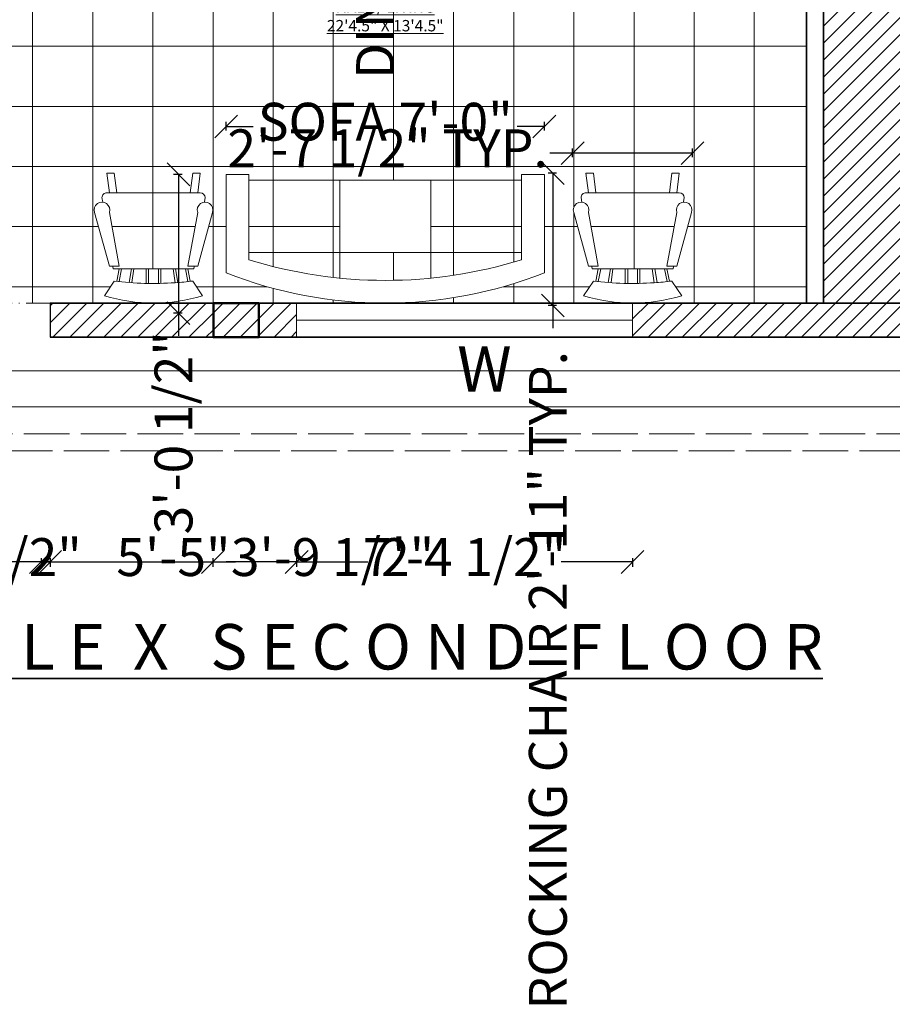
# Model space of a CAD drawing. Units: inches. Extents: x 2036 to 2670, y 319 to 920.
# Tile 2 of 15: x 2219 to 2449, y 319 to 579. Entities that reach past the tile are written whole.
import ezdxf

# ---------------------------------------------------------------- set-up
doc = ezdxf.new("R2010")
doc.units = ezdxf.units.IN
doc.linetypes.add('ACAD_ISO02W100', pattern=[15, 12, -3])
doc.linetypes.add('ACAD_ISO06W100', pattern=[36, 24, -3, 0, -3, 0, -3, 0, -3])
for name, color, linetype, lineweight in [('A-ANNO-DIMS', 2, 'Continuous', 18), ('A-ANNO-TEXT', 7, 'Continuous', 18), ('A-ANNO-TITL', 7, 'Continuous', 35), ('A-AREA-IDEN', 7, 'Continuous', 18), ('A-CASE-PATT', 9, 'Continuous', 13), ('A-COLS', 7, 'Continuous', 50), ('A-DOOR', 3, 'Continuous', 25), ('A-DOOR-OVHD', 3, 'ACAD_ISO06W100', 18), ('A-FLOR-OVHD', 1, 'ACAD_ISO02W100', 13), ('A-FLOR-PATT', 8, 'Continuous', 9), ('A-FURN', 8, 'Continuous', 18), ('A-GLAZ', 4, 'Continuous', 18), ('A-WALL', 7, 'Continuous', 35)]:
    doc.layers.add(name, color=color, linetype=linetype, lineweight=lineweight)
doc.layers.add('A-COLS-PATT', color=240, linetype='Continuous', lineweight=13, true_color=0xed1f24)
doc.layers.add('A-WALL-PATT', color=52, linetype='Continuous', lineweight=13, true_color=0xc8c92d)
doc.styles.get("Standard").update_dxf_attribs({"font": 'arial.ttf'})
doc.dimstyles.new('ISO-25', dxfattribs={"dimtxt": 10, "dimasz": 6, "dimexe": 1.25, "dimexo": 0.625, "dimtad": 0, "dimdec": 1, "dimlunit": 3, "dimtxsty": 'Standard', "dimblk": 'OBLIQUE', "dimcen": 2.5, "dimclrd": 94, "dimclre": 94, "dimclrt": 1, "dimadec": 0, "dimazin": 0, "dimtfac": 1, "dimtdec": 1, "dimtmove": 0, "dimatfit": 3, "dimfxl": 1, "dimfxlon": 1, "dimarcsym": 0})

# ---------------------------------------------------------------- blocks, each defined once
blk = doc.blocks.new('Chair - Rocking')
for p, q in [((-8, -4.5), (-10, -1.5)), ((8, -4.5), (10, -1.5)), ((-7.5, -4.5), (-7, -7)), ((-6.5, -7), (-7.02225, -4.43)), ((-4.5, -7), (-4.96674, -4.19951)), ((-4, -7), (-4.40532, -4.16272)), ((-1.5, -4.05012), (-1.5, -7)), ((-1, -7), (-1, -4.05012)), ((1, -7), (1, -4.04655)), ((1.5, -4.05012), (1.5, -7)), ((4, -7), (4.40187, -4.18694)), ((4.5, -7), (4.96761, -4.19437)), ((6.5, -7), (7, -4.4057)), ((7.5, -4.5), (7, -7)), ((-9, -7.5), (-12, -18.49999)), ((-7, -7.5), (-9, -7.5)), ((-9, -18.49999), (-7, -7.5)), ((-8.23428, -6.99939), (-8.3093, -7.47958)), ((-8.23041, -7), (8.23915, -7)), ((7, -7.5), (9, -7.5)), ((9, -18.49999), (7, -7.5)), ((8.31071, -7.48854), (8.23449, -7.00073)), ((9, -7.5), (12, -18.49999)), ((-10.36644, -20.64523), (-10.5, -21.49999)), ((10.5, -21.49999), (10.3575, -20.58798)), ((-9, -22.49999), (-9.5, -26.49999)), ((0, -22.49999), (-9.5, -22.49999)), ((-8, -26.49999), (-7.5, -22.49999)), ((0, -22.49999), (9.5, -22.49999)), ((8, -26.49999), (7.5, -22.49999)), ((9, -22.49999), (9.5, -26.49999)), ((-9.5, -26.49999), (-8, -26.49999)), ((9.5, -26.49999), (8, -26.49999))]:
    blk.add_line(p, q)
for centre, radius, start, end in [((0, -34.08333), 34.08333, 72.93847, 107.0615), ((0, -68.25004), 64.25, 82.84733, 93.92211), ((0, -68.25004), 64.25, 93.92211, 97.15267), ((-10.5, -18.99999), 1.58114, 161.5651, 18.43495), ((10.5, -18.99999), 1.58114, 161.5651, 18.43495), ((-9.5, -21.49999), 1, 180, 270), ((9.5, -21.49999), 1, 270, 0)]:
    blk.add_arc(centre, radius, start, end)
blk = doc.blocks.new('Sofa - Roundback 7 ft.')
for p, q in [((-12.00002, -32.4421), (-12.00003, -6.5971)), ((11.99997, -32.4421), (11.99998, -6.5971)), ((-36.000027, -34), (-36.000027, -11.4696)), ((35.99998, -34), (35.99998, -11.4696)), ((-35.999844, -13.3819), (35.9998, -13.3819)), ((-36.000027, -32.4421), (35.99998, -32.4421))]:
    blk.add_line(p, q)
for points in [[(-36.000027, -34), (-42.000027, -34), (-42.000027, -8)], [(41.99998, -8), (41.99998, -34), (35.99998, -34)]]:
    blk.add_lwpolyline(points)
for centre, radius, start, end in [((0, -114.25), 114.25, 68.43141, 111.5686), ((-0.00001, -127.1968), 121.1968, 72.72033, 107.2797)]:
    blk.add_arc(centre, radius, start, end)
blk = doc.blocks.new('COL-9x12')
blk.add_lwpolyline([(9, 0), (0, 0), (0, 12), (9, 12)], close=True)
blk = doc.blocks.new('_Oblique')
at = {"color": 0, "linetype": 'ByBlock', "lineweight": -2}
blk.add_line((-0.5, -0.5), (0.5, 0.5), dxfattribs=at)
blk = doc.blocks.new('*D25')
at = {"layer": 'A-ANNO-DIMS', "color": 94, "lineweight": -2, "transparency": 16777216}
for p, q in [((2360.81, 538.02), (2358.56, 538.02)), ((2359.81, 538.02), (2359.81, 503.04)), ((2360.81, 503.04), (2358.56, 503.04)), ((2359.81, 503.04), (2359.81, 497.04))]:
    blk.add_line(p, q, dxfattribs=at)
at = {"layer": 'Defpoints', "color": 0, "transparency": 16777216}
for p in [(2365.06, 538.02), (2359.81, 503.04), (2365.06, 503.04)]:
    blk.add_point(p, dxfattribs=at)
at = {"layer": 'A-ANNO-DIMS', "color": 94, "lineweight": -2, "transparency": 16777216, "xscale": 6, "yscale": 6, "zscale": 6}
for p, rotation in [((2359.81, 538.02), 90), ((2359.81, 503.04), 270)]:
    blk.add_blockref('_Oblique', p, dxfattribs=dict(at, rotation=rotation))
at = {"layer": 'A-ANNO-DIMS', "color": 1, "transparency": 16777216, "insert": (2359.81, 404.1), "char_height": 10, "attachment_point": 5, "rotation": 90}
blk.add_mtext('ROCKING CHAIR 2\'-11" TYP.', dxfattribs=at)
blk = doc.blocks.new('*D26')
at = {"layer": 'A-ANNO-DIMS', "color": 94, "lineweight": -2, "transparency": 16777216}
for p, q in [((2365.06, 542.26), (2365.06, 544.51)), ((2396.72, 542.26), (2396.72, 544.51)), ((2365.06, 543.26), (2359.06, 543.26)), ((2396.72, 543.26), (2365.06, 543.26))]:
    blk.add_line(p, q, dxfattribs=at)
at = {"layer": 'Defpoints', "color": 0, "transparency": 16777216}
for p in [(2365.06, 543.26), (2365.06, 538.02), (2396.72, 538.02)]:
    blk.add_point(p, dxfattribs=at)
at = {"layer": 'A-ANNO-DIMS', "color": 94, "lineweight": -2, "transparency": 16777216, "xscale": 6, "yscale": 6, "zscale": 6, "rotation": 180}
blk.add_blockref('_Oblique', (2365.06, 543.26), dxfattribs=at)
at = {"layer": 'A-ANNO-DIMS', "color": 94, "lineweight": -2, "transparency": 16777216, "xscale": 6, "yscale": 6, "zscale": 6}
blk.add_blockref('_Oblique', (2396.72, 543.26), dxfattribs=at)
at = {"layer": 'A-ANNO-DIMS', "color": 1, "transparency": 16777216, "insert": (2316.22, 543.26), "char_height": 10, "attachment_point": 5}
blk.add_mtext('2\'-7 1/2" TYP.', dxfattribs=at)
blk = doc.blocks.new('*D33')
at = {"layer": 'A-ANNO-DIMS', "color": 94, "lineweight": -2, "transparency": 16777216}
for p, q in [((2273.59, 549.28), (2273.59, 551.53)), ((2357.59, 549.28), (2357.59, 551.53)), ((2273.59, 550.28), (2280.74, 550.28)), ((2357.59, 550.28), (2350.44, 550.28))]:
    blk.add_line(p, q, dxfattribs=at)
at = {"layer": 'Defpoints', "color": 0, "transparency": 16777216}
for p in [(2273.59, 550.28), (2273.59, 537.68), (2357.59, 537.68)]:
    blk.add_point(p, dxfattribs=at)
at = {"layer": 'A-ANNO-DIMS', "color": 94, "lineweight": -2, "transparency": 16777216, "xscale": 6, "yscale": 6, "zscale": 6, "rotation": 180}
blk.add_blockref('_Oblique', (2273.59, 550.28), dxfattribs=at)
at = {"layer": 'A-ANNO-DIMS', "color": 94, "lineweight": -2, "transparency": 16777216, "xscale": 6, "yscale": 6, "zscale": 6}
blk.add_blockref('_Oblique', (2357.59, 550.28), dxfattribs=at)
at = {"layer": 'A-ANNO-DIMS', "color": 1, "transparency": 16777216, "insert": (2315.59, 550.28), "char_height": 10, "attachment_point": 5}
blk.add_mtext('SOFA 7\'-0"', dxfattribs=at)
blk = doc.blocks.new('*D34')
at = {"layer": 'A-ANNO-DIMS', "color": 94, "lineweight": -2, "transparency": 16777216}
for p, q in [((2261.99, 537.68), (2259.74, 537.68)), ((2260.99, 537.68), (2260.99, 501.02)), ((2261.99, 501.02), (2259.74, 501.02)), ((2260.99, 501.02), (2260.99, 495.02))]:
    blk.add_line(p, q, dxfattribs=at)
at = {"layer": 'Defpoints', "color": 0, "transparency": 16777216}
for p in [(2273.59, 537.68), (2260.99, 501.02), (2273.59, 501.02)]:
    blk.add_point(p, dxfattribs=at)
at = {"layer": 'A-ANNO-DIMS', "color": 94, "lineweight": -2, "transparency": 16777216, "xscale": 6, "yscale": 6, "zscale": 6}
for p, rotation in [((2260.99, 537.68), 90), ((2260.99, 501.02), 270)]:
    blk.add_blockref('_Oblique', p, dxfattribs=dict(at, rotation=rotation))
at = {"layer": 'A-ANNO-DIMS', "color": 1, "transparency": 16777216, "insert": (2260.99, 469.45), "char_height": 10, "attachment_point": 5, "rotation": 90}
blk.add_mtext('3\'-0 1/2"', dxfattribs=at)
blk = doc.blocks.new('*D39')
at = {"layer": 'A-ANNO-DIMS', "color": 94, "lineweight": -2, "transparency": 16777216}
for p, q in [((2315.21, 769.01), (2312.96, 769.01)), ((2314.21, 769.01), (2314.21, 678.01)), ((2315.21, 678.01), (2312.96, 678.01)), ((2314.21, 678.01), (2314.21, 672.01))]:
    blk.add_line(p, q, dxfattribs=at)
at = {"layer": 'Defpoints', "color": 0, "transparency": 16777216}
for p in [(2327.86, 769.01), (2314.21, 678.01), (2327.86, 678.01)]:
    blk.add_point(p, dxfattribs=at)
at = {"layer": 'A-ANNO-DIMS', "color": 94, "lineweight": -2, "transparency": 16777216, "xscale": 6, "yscale": 6, "zscale": 6}
for p, rotation in [((2314.21, 769.01), 90), ((2314.21, 678.01), 270)]:
    blk.add_blockref('_Oblique', p, dxfattribs=dict(at, rotation=rotation))
at = {"layer": 'A-ANNO-DIMS', "color": 1, "transparency": 16777216, "insert": (2314.21, 616.43), "char_height": 10, "attachment_point": 5, "rotation": 90}
blk.add_mtext('DINING SET 7\'-7"', dxfattribs=at)
blk = doc.blocks.new('*D41')
at = {"layer": 'A-ANNO-DIMS', "color": 94, "lineweight": -2, "transparency": 16777216}
for p, q in [((2149.74, 436.33), (2149.74, 434.08)), ((2149.74, 435.33), (2177.02, 435.33)), ((2177.02, 436.33), (2177.02, 434.08)), ((2177.02, 435.33), (2183.02, 435.33))]:
    blk.add_line(p, q, dxfattribs=at)
at = {"layer": 'Defpoints', "color": 0, "transparency": 16777216}
for p in [(2149.74, 494.68), (2177.02, 494.68), (2177.02, 435.33)]:
    blk.add_point(p, dxfattribs=at)
at = {"layer": 'A-ANNO-DIMS', "color": 94, "lineweight": -2, "transparency": 16777216, "xscale": 6, "yscale": 6, "zscale": 6, "rotation": 180}
blk.add_blockref('_Oblique', (2149.74, 435.33), dxfattribs=at)
at = {"layer": 'A-ANNO-DIMS', "color": 94, "lineweight": -2, "transparency": 16777216, "xscale": 6, "yscale": 6, "zscale": 6}
blk.add_blockref('_Oblique', (2177.02, 435.33), dxfattribs=at)
at = {"layer": 'A-ANNO-DIMS', "color": 1, "transparency": 16777216, "insert": (2208.67, 435.33), "char_height": 10, "attachment_point": 5}
blk.add_mtext('2\'-3 1/2"', dxfattribs=at)
blk = doc.blocks.new('*D42')
at = {"layer": 'A-ANNO-DIMS', "color": 94, "lineweight": -2, "transparency": 16777216}
for p, q in [((2177.02, 436.33), (2177.02, 434.08)), ((2177.02, 435.33), (2187.98, 435.33)), ((2227.17, 435.33), (2216.21, 435.33)), ((2227.17, 436.33), (2227.17, 434.08))]:
    blk.add_line(p, q, dxfattribs=at)
at = {"layer": 'Defpoints', "color": 0, "transparency": 16777216}
for p in [(2177.02, 494.68), (2227.17, 494.68), (2227.17, 435.33)]:
    blk.add_point(p, dxfattribs=at)
at = {"layer": 'A-ANNO-DIMS', "color": 94, "lineweight": -2, "transparency": 16777216, "xscale": 6, "yscale": 6, "zscale": 6, "rotation": 180}
blk.add_blockref('_Oblique', (2177.02, 435.33), dxfattribs=at)
at = {"layer": 'A-ANNO-DIMS', "color": 94, "lineweight": -2, "transparency": 16777216, "xscale": 6, "yscale": 6, "zscale": 6}
blk.add_blockref('_Oblique', (2227.17, 435.33), dxfattribs=at)
at = {"layer": 'A-ANNO-DIMS', "color": 1, "transparency": 16777216, "insert": (2202.09, 435.33), "char_height": 10, "attachment_point": 5}
blk.add_mtext('4\'-2"', dxfattribs=at)
blk = doc.blocks.new('*D43')
at = {"layer": 'A-ANNO-DIMS', "color": 94, "lineweight": -2, "transparency": 16777216}
for p, q in [((2227.17, 436.33), (2227.17, 434.08)), ((2227.17, 435.33), (2245.77, 435.33)), ((2292.21, 435.33), (2273.61, 435.33)), ((2292.21, 436.33), (2292.21, 434.08))]:
    blk.add_line(p, q, dxfattribs=at)
at = {"layer": 'Defpoints', "color": 0, "transparency": 16777216}
for p in [(2227.17, 494.68), (2292.21, 494.68), (2292.21, 435.33)]:
    blk.add_point(p, dxfattribs=at)
at = {"layer": 'A-ANNO-DIMS', "color": 94, "lineweight": -2, "transparency": 16777216, "xscale": 6, "yscale": 6, "zscale": 6, "rotation": 180}
blk.add_blockref('_Oblique', (2227.17, 435.33), dxfattribs=at)
at = {"layer": 'A-ANNO-DIMS', "color": 94, "lineweight": -2, "transparency": 16777216, "xscale": 6, "yscale": 6, "zscale": 6}
blk.add_blockref('_Oblique', (2292.21, 435.33), dxfattribs=at)
at = {"layer": 'A-ANNO-DIMS', "color": 1, "transparency": 16777216, "insert": (2259.69, 435.33), "char_height": 10, "attachment_point": 5}
blk.add_mtext('5\'-5"', dxfattribs=at)
blk = doc.blocks.new('*D44')
at = {"layer": 'A-ANNO-DIMS', "color": 94, "lineweight": -2, "transparency": 16777216}
for p, q in [((2292.21, 436.33), (2292.21, 434.08)), ((2292.21, 435.33), (2311.02, 435.33)), ((2380.89, 435.33), (2362.07, 435.33)), ((2380.89, 436.33), (2380.89, 434.08))]:
    blk.add_line(p, q, dxfattribs=at)
at = {"layer": 'Defpoints', "color": 0, "transparency": 16777216}
for p in [(2292.21, 494.68), (2380.89, 494.68), (2380.89, 435.33)]:
    blk.add_point(p, dxfattribs=at)
at = {"layer": 'A-ANNO-DIMS', "color": 94, "lineweight": -2, "transparency": 16777216, "xscale": 6, "yscale": 6, "zscale": 6, "rotation": 180}
blk.add_blockref('_Oblique', (2292.21, 435.33), dxfattribs=at)
at = {"layer": 'A-ANNO-DIMS', "color": 94, "lineweight": -2, "transparency": 16777216, "xscale": 6, "yscale": 6, "zscale": 6}
blk.add_blockref('_Oblique', (2380.89, 435.33), dxfattribs=at)
at = {"layer": 'A-ANNO-DIMS', "color": 1, "transparency": 16777216, "insert": (2336.55, 435.33), "char_height": 10, "attachment_point": 5}
blk.add_mtext('7\'-4 1/2"', dxfattribs=at)
blk = doc.blocks.new('*D54')
at = {"layer": 'A-ANNO-DIMS', "color": 94, "lineweight": -2, "transparency": 16777216}
for p, q in [((2642.09, 545.51), (2642.09, 551.51)), ((2641.09, 545.51), (2643.34, 545.51)), ((2642.09, 513.19), (2642.09, 545.51)), ((2641.09, 513.19), (2643.34, 513.19))]:
    blk.add_line(p, q, dxfattribs=at)
at = {"layer": 'Defpoints', "color": 0, "transparency": 16777216}
for p in [(2158.74, 545.51), (2642.09, 545.51), (2158.74, 513.19)]:
    blk.add_point(p, dxfattribs=at)
at = {"layer": 'A-ANNO-DIMS', "color": 94, "lineweight": -2, "transparency": 16777216, "xscale": 6, "yscale": 6, "zscale": 6}
for p, rotation in [((2642.09, 545.51), 90), ((2642.09, 513.19), 270)]:
    blk.add_blockref('_Oblique', p, dxfattribs=dict(at, rotation=rotation))
at = {"layer": 'A-ANNO-DIMS', "color": 1, "transparency": 16777216, "insert": (2642.09, 577.16), "char_height": 10, "attachment_point": 5, "rotation": 90}
blk.add_mtext('2\'-8 1/2"', dxfattribs=at)
blk = doc.blocks.new('*D55')
at = {"layer": 'A-ANNO-DIMS', "color": 94, "lineweight": -2, "transparency": 16777216}
for p, q in [((2641.09, 582.53), (2643.34, 582.53)), ((2642.09, 582.53), (2642.09, 577.94)), ((2642.09, 545.51), (2642.09, 550.11)), ((2641.09, 545.51), (2643.34, 545.51))]:
    blk.add_line(p, q, dxfattribs=at)
at = {"layer": 'Defpoints', "color": 0, "transparency": 16777216}
for p in [(2158.74, 582.53), (2642.09, 582.53), (2158.74, 545.51)]:
    blk.add_point(p, dxfattribs=at)
at = {"layer": 'A-ANNO-DIMS', "color": 94, "lineweight": -2, "transparency": 16777216, "xscale": 6, "yscale": 6, "zscale": 6}
for p, rotation in [((2642.09, 582.53), 90), ((2642.09, 545.51), 270)]:
    blk.add_blockref('_Oblique', p, dxfattribs=dict(at, rotation=rotation))
at = {"layer": 'A-ANNO-DIMS', "color": 1, "transparency": 16777216, "insert": (2642.09, 564.02), "char_height": 10, "attachment_point": 5, "rotation": 90}
blk.add_mtext('3\'-1"', dxfattribs=at)
blk = doc.blocks.new('*D58')
at = {"layer": 'A-ANNO-DIMS', "color": 94, "lineweight": -2, "transparency": 16777216}
for p, q in [((2224.74, 436.33), (2224.74, 434.08)), ((2224.74, 435.33), (2270.11, 435.33)), ((2270.11, 436.33), (2270.11, 434.08)), ((2270.11, 435.33), (2276.11, 435.33))]:
    blk.add_line(p, q, dxfattribs=at)
at = {"layer": 'Defpoints', "color": 0, "transparency": 16777216}
for p in [(2224.74, 824.68), (2270.11, 824.68), (2270.11, 435.33)]:
    blk.add_point(p, dxfattribs=at)
at = {"layer": 'A-ANNO-DIMS', "color": 94, "lineweight": -2, "transparency": 16777216, "xscale": 6, "yscale": 6, "zscale": 6, "rotation": 180}
blk.add_blockref('_Oblique', (2224.74, 435.33), dxfattribs=at)
at = {"layer": 'A-ANNO-DIMS', "color": 94, "lineweight": -2, "transparency": 16777216, "xscale": 6, "yscale": 6, "zscale": 6}
blk.add_blockref('_Oblique', (2270.11, 435.33), dxfattribs=at)
at = {"layer": 'A-ANNO-DIMS', "color": 1, "transparency": 16777216, "insert": (2301.68, 435.33), "char_height": 10, "attachment_point": 5}
blk.add_mtext('3\'-9 1/2"', dxfattribs=at)
blk = doc.blocks.new('*D60')
at = {"layer": 'A-ANNO-DIMS', "color": 94, "lineweight": -2, "transparency": 16777216}
for p, q in [((2051.39, 582.41), (2051.39, 588.41)), ((2052.39, 582.41), (2050.14, 582.41)), ((2051.39, 545.09), (2051.39, 582.41)), ((2052.39, 545.09), (2050.14, 545.09))]:
    blk.add_line(p, q, dxfattribs=at)
at = {"layer": 'Defpoints', "color": 0, "transparency": 16777216}
for p in [(2051.39, 582.41), (2515.24, 582.41), (2515.24, 545.09)]:
    blk.add_point(p, dxfattribs=at)
at = {"layer": 'A-ANNO-DIMS', "color": 94, "lineweight": -2, "transparency": 16777216, "xscale": 6, "yscale": 6, "zscale": 6}
for p, rotation in [((2051.39, 582.41), 90), ((2051.39, 545.09), 270)]:
    blk.add_blockref('_Oblique', p, dxfattribs=dict(at, rotation=rotation))
at = {"layer": 'A-ANNO-DIMS', "color": 1, "transparency": 16777216, "insert": (2051.39, 613.98), "char_height": 10, "attachment_point": 5, "rotation": 90}
blk.add_mtext('3\'-1 1/2"', dxfattribs=at)

msp = doc.modelspace()

# ---------------------------------------------------------------- hatches: boundary and pattern name
at = {"layer": 'A-CASE-PATT'}
h = msp.add_hatch(dxfattribs=at)
h.set_pattern_fill('ANSI31', color=256)
h.paths.add_polyline_path([(2455.24, 614.68), (2431.24, 614.68), (2431.24, 503.68), (2515.24, 503.68), (2515.24, 527.68), (2455.24, 527.68)])
at = {"layer": 'A-COLS-PATT'}
h = msp.add_hatch(dxfattribs=at)
h.set_pattern_fill('ANSI31', color=256)
h.paths.add_polyline_path([(2089.74, 875.68), (2080.74, 875.68), (2080.74, 863.68), (2089.74, 863.68)])
h.paths.add_polyline_path([(2089.74, 821.68), (2080.74, 821.68), (2080.74, 809.68), (2089.74, 809.68)])
h.paths.add_polyline_path([(2089.74, 624.2), (2080.74, 624.2), (2080.74, 612.2), (2089.74, 612.2)])
h.paths.add_polyline_path([(2158.74, 506.68), (2149.74, 506.68), (2149.74, 494.68), (2158.74, 494.68)])
h.paths.add_polyline_path([(2158.74, 617.33), (2149.74, 617.33), (2149.74, 605.33), (2158.74, 605.33)])
h.paths.add_polyline_path([(2158.74, 736.18), (2149.74, 736.18), (2149.74, 724.18), (2158.74, 724.18)])
h.paths.add_polyline_path([(2158.74, 852.81), (2149.74, 852.81), (2149.74, 843.81), (2158.74, 843.81)])
h.paths.add_polyline_path([(2161.74, 852.81), (2158.74, 852.81), (2158.74, 843.81), (2161.74, 843.81)])
h.paths.add_polyline_path([(2295.21, 857.66), (2290.74, 857.66), (2290.74, 848.68), (2295.21, 848.68)])
h.paths.add_polyline_path([(2290.74, 857.66), (2283.21, 857.66), (2283.21, 848.66), (2290.74, 848.66)])
h.paths.add_polyline_path([(2443.62, 857.68), (2431.62, 857.68), (2431.62, 848.68), (2443.62, 848.68)])
h.paths.add_polyline_path([(2561.81, 857.68), (2549.81, 857.68), (2549.81, 848.68), (2561.81, 848.68)])
h.paths.add_polyline_path([(2295.24, 737.65), (2290.74, 737.65), (2290.74, 728.68), (2295.24, 728.68)])
h.paths.add_polyline_path([(2309.27, 612.12), (2297.27, 612.12), (2297.27, 603.12), (2309.27, 603.12)])
h.paths.add_polyline_path([(2282.24, 503.68), (2270.24, 503.68), (2270.24, 494.68), (2282.24, 494.68)])
h.paths.add_polyline_path([(2431.74, 746.09), (2427.24, 746.09), (2427.24, 737.09), (2431.74, 737.09)])
h.paths.add_polyline_path([(2439.24, 746.09), (2431.74, 746.09), (2431.74, 737.09), (2439.24, 737.09)])
h.paths.add_polyline_path([(2596.59, 736.59), (2584.59, 736.59), (2584.59, 727.59), (2596.59, 727.59)])
h.paths.add_polyline_path([(2586.39, 623.71), (2574.39, 623.71), (2574.39, 619.18), (2586.39, 619.18)])
h.paths.add_polyline_path([(2586.39, 619.18), (2574.39, 619.18), (2574.39, 614.71), (2586.39, 614.71)])
h.paths.add_polyline_path([(2438.74, 623.68), (2431.24, 623.68), (2431.24, 619.18), (2438.74, 619.18)])
h.paths.add_polyline_path([(2438.74, 619.18), (2431.24, 619.18), (2431.24, 614.68), (2438.74, 614.68)])
h.paths.add_polyline_path([(2431.24, 623.68), (2426.74, 623.68), (2426.74, 614.68), (2431.24, 614.68), (2431.24, 619.18)])
h.paths.add_polyline_path([(2527.24, 503.68), (2515.24, 503.68), (2515.24, 494.68), (2527.24, 494.68)])
h.paths.add_polyline_path([(2590.31, 503.68), (2578.31, 503.68), (2578.31, 494.68), (2590.31, 494.68)])
at = {"layer": 'A-FLOR-PATT'}
h = msp.add_hatch(dxfattribs=at)
h.set_pattern_fill('ANSI31', color=256, scale=5, angle=135)
h.paths.add_polyline_path([(2290.74, 659.68), (2158.74, 659.68), (2158.74, 582.53), (2158.74, 545.51), (2158.74, 503.68), (2426.74, 503.68), (2426.74, 614.68), (2426.74, 623.68), (2426.74, 628.18), (2431.24, 628.18), (2431.24, 623.68), (2438.74, 623.68), (2438.74, 619.18), (2574.39, 619.18), (2574.39, 623.71), (2586.39, 623.71), (2586.39, 619.18), (2603.74, 619.18), (2603.74, 824.68), (2431.74, 824.68), (2431.74, 746.09), (2439.24, 746.09), (2439.24, 737.09), (2431.74, 737.09), (2431.74, 659.68), (2427.24, 659.68), (2427.24, 739.48), (2383.24, 739.48), (2383.24, 804.68), (2339.24, 804.68), (2339.24, 749.08), (2295.24, 749.08), (2295.24, 737.65), (2295.27, 737.65), (2295.27, 728.65), (2295.21, 728.65, -0.586418), (2272.74, 728.68), (2272.74, 824.68), (2270.11, 824.68), (2270.11, 829.18), (2290.74, 829.18), (2290.74, 848.66), (2283.21, 848.66), (2283.21, 857.66), (2289.74, 857.66), (2289.74, 874.68), (2158.74, 874.68), (2158.74, 852.81), (2161.74, 852.81), (2161.74, 843.81), (2158.74, 843.81), (2158.74, 829.18), (2224.74, 829.18), (2224.74, 800.68), (2182.74, 800.68), (2182.74, 733.41), (2158.74, 733.41), (2158.74, 728.68), (2235.24, 728.68), (2235.24, 714.81), (2230.74, 714.81), (2230.74, 724.18), (2158.74, 724.18), (2158.74, 664.18), (2230.74, 664.18), (2230.74, 678.81), (2235.24, 678.81), (2235.24, 664.18), (2290.74, 664.18)])
h.paths.add_polyline_path([(2309.27, 612.12), (2309.27, 603.12), (2297.27, 603.12), (2297.27, 612.12)], flags=16)
h.paths.add_polyline_path([(2280.12, 639.11), (2280.26, 638.18, -0.414214), (2279.26, 637.18), (2278.76, 637.18), (2279.26, 633.18), (2277.76, 633.18), (2277.26, 637.18), (2269.76, 637.18), (2262.26, 637.18), (2261.76, 633.18), (2260.26, 633.18), (2260.76, 637.18), (2260.26, 637.18, -0.414214), (2259.26, 638.18), (2259.41, 639.11, -0.541164), (2257.76, 641.18), (2260.76, 652.18), (2261.45, 652.18), (2261.53, 652.68), (2262.76, 652.68), (2262.25, 655.24, 0.001913), (2261.76, 655.18), (2259.76, 658.18, -0.15), (2279.76, 658.18), (2277.76, 655.18, 0.001913), (2277.27, 655.24), (2276.76, 652.68), (2278, 652.68), (2278.07, 652.18), (2278.76, 652.18), (2281.76, 641.18, -0.541163)], flags=16)
h.paths.add_polyline_path([(2245.98, 639.11), (2246.13, 638.18, -0.414214), (2245.13, 637.18), (2244.63, 637.18), (2245.13, 633.18), (2243.63, 633.18), (2243.13, 637.18), (2235.63, 637.18), (2228.13, 637.18), (2227.63, 633.18), (2226.13, 633.18), (2226.63, 637.18), (2226.13, 637.18, -0.414214), (2225.13, 638.18), (2225.27, 639.11, -0.541164), (2223.63, 641.18), (2226.63, 652.18), (2227.32, 652.18), (2227.39, 652.68), (2228.63, 652.68), (2228.12, 655.24, 0.001913), (2227.63, 655.18), (2225.63, 658.18, -0.15), (2245.63, 658.18), (2243.63, 655.18, 0.001913), (2243.14, 655.24), (2242.63, 652.68), (2243.86, 652.68), (2243.94, 652.18), (2244.63, 652.18), (2247.63, 641.18, -0.541163)], flags=16)
h.paths.add_polyline_path([(2351.59, 515.15, -0.151948), (2279.59, 515.15), (2279.59, 537.68), (2273.59, 537.68), (2273.59, 511.68, 0.190476), (2357.59, 511.68), (2357.59, 537.68), (2351.59, 537.68)])
h.paths.add_polyline_path([(2327.59, 536.13), (2327.59, 517.07), (2303.59, 517.07), (2303.59, 536.13)], flags=16)
h.paths.add_polyline_path([(2213.4, 639.11), (2213.55, 638.18, -0.414214), (2212.55, 637.18), (2212.05, 637.18), (2212.55, 633.18), (2211.05, 633.18), (2210.55, 637.18), (2203.05, 637.18), (2195.55, 637.18), (2195.05, 633.18), (2193.55, 633.18), (2194.05, 637.18), (2193.55, 637.18, -0.414214), (2192.55, 638.18), (2192.69, 639.11, -0.541164), (2191.05, 641.18), (2194.05, 652.18), (2194.73, 652.18), (2194.81, 652.68), (2196.05, 652.68), (2195.53, 655.24, 0.001913), (2195.05, 655.18), (2193.05, 658.18, -0.15), (2213.05, 658.18), (2211.05, 655.18, 0.001913), (2210.56, 655.24), (2210.05, 652.68), (2211.28, 652.68), (2211.36, 652.18), (2212.05, 652.18), (2215.05, 641.18, -0.541163)], flags=16)
h.paths.add_polyline_path([(2368.58, 538.02), (2370.52, 538.02), (2371.17, 532.84), (2380.89, 532.84), (2390.6, 532.84), (2391.25, 538.02), (2393.2, 538.02), (2392.55, 532.84), (2380.89, 532.84), (2368.58, 532.84, 0.414214), (2367.28, 531.54), (2367.47, 530.34, -0.483352), (2369.23, 527.65), (2371.82, 513.4), (2370.12, 513.4), (2370.22, 512.75), (2391.56, 512.75), (2391.66, 513.4), (2389.96, 513.4), (2392.55, 527.65, -1.387427), (2396.43, 527.65), (2392.55, 513.4), (2391.66, 513.4), (2391.56, 512.75), (2389.31, 512.75), (2390, 509.37, 0.003796), (2391.25, 509.51), (2393.84, 505.63, -0.15), (2367.93, 505.63), (2370.52, 509.51, 0.003901), (2371.81, 509.36), (2372.47, 512.75), (2370.22, 512.75), (2370.12, 513.4), (2369.23, 513.4), (2365.34, 527.65, -0.541163), (2367.47, 530.34), (2367.28, 531.54, -0.414214), (2368.58, 532.84), (2369.23, 532.84)])
h.paths.add_polyline_path([(2266.74, 538.02), (2266.09, 532.84), (2254.43, 532.84), (2242.12, 532.84, 0.414214), (2240.83, 531.54), (2241.01, 530.34, -0.483352), (2242.77, 527.65), (2245.36, 513.4), (2243.66, 513.4), (2243.76, 512.75), (2265.1, 512.75), (2265.2, 513.4), (2263.5, 513.4), (2266.09, 527.65, -1.387427), (2269.98, 527.65), (2266.09, 513.4), (2265.2, 513.4), (2265.1, 512.75), (2262.85, 512.75), (2263.54, 509.37, 0.003796), (2264.79, 509.51), (2267.39, 505.63, -0.15), (2241.47, 505.63), (2244.07, 509.51, 0.003901), (2245.36, 509.36), (2246.01, 512.75), (2243.76, 512.75), (2243.66, 513.4), (2242.77, 513.4), (2238.88, 527.65, -0.541163), (2241.01, 530.34), (2240.83, 531.54, -0.414214), (2242.12, 532.84), (2242.77, 532.84), (2242.12, 538.02), (2244.07, 538.02), (2244.71, 532.84), (2254.43, 532.84), (2264.15, 532.84), (2264.79, 538.02)])
h.paths.add_polyline_path([(2185.24, 620.36), (2185.24, 618.86), (2181.24, 618.36), (2181.24, 610.86), (2181.24, 603.36), (2185.24, 602.86), (2185.24, 601.36), (2181.24, 601.86), (2181.24, 601.36, -0.414214), (2180.24, 600.36), (2179.31, 600.5, -0.541164), (2177.24, 598.86), (2166.24, 601.86), (2166.24, 602.54), (2165.74, 602.62), (2165.74, 603.86), (2163.18, 603.34, 0.001913), (2163.24, 602.86), (2160.24, 600.86, -0.15), (2160.24, 620.86), (2163.24, 618.86, 0.001913), (2163.18, 618.37), (2165.74, 617.86), (2165.74, 619.09), (2166.24, 619.17), (2166.24, 619.86), (2177.24, 622.86, -0.541163), (2179.31, 621.21), (2180.24, 621.36, -0.414214), (2181.24, 620.36), (2181.24, 619.86)])
h.paths.add_polyline_path([(2470.92, 676.01), (2470.92, 806.13), (2568.52, 806.13), (2568.52, 676.01)], flags=16)
h.paths.add_polyline_path([(2177.74, 677.49), (2161.9, 677.49), (2161.9, 705.85), (2177.74, 705.85)], flags=16)
h.paths.add_polyline_path([(2176.74, 678.49), (2162.9, 678.49), (2162.9, 704.85), (2176.74, 704.85)], flags=0)
h.paths.add_polyline_path([(2175.01, 686.48), (2172.93, 686.48), (2172.93, 690.63), (2170.86, 690.63), (2170.86, 686.48), (2164.63, 686.48), (2164.63, 688.56), (2166.71, 688.56), (2168.78, 688.56), (2168.78, 690.63), (2164.63, 690.63), (2164.63, 696.85), (2166.71, 696.85), (2166.71, 692.71), (2168.78, 692.71), (2168.78, 696.85), (2175.01, 696.85), (2175.01, 694.78), (2170.86, 694.78), (2170.86, 692.71), (2175.01, 692.71)], flags=0)
h.paths.add_polyline_path([(2543.79, 782.71), (2483.94, 782.71), (2483.94, 804.18), (2517.77, 804.18), (2517.77, 782.71), (2521.67, 782.71), (2521.67, 804.18), (2555.5, 804.18), (2555.5, 779.45), (2547.05, 779.45), (2568.52, 757.98), (2543.79, 757.98)], flags=0)
h.paths.add_polyline_path([(2584.59, 727.59), (2584.59, 736.59), (2596.59, 736.59), (2596.59, 727.59)], flags=16)
h.paths.add_polyline_path([(2520.45, 647.03), (2553.79, 647.03), (2553.79, 658.23), (2520.45, 658.23)], flags=24)
h.paths.add_polyline_path([(2299.53, 573.74), (2331.71, 573.74), (2331.71, 584.94), (2299.53, 584.94)], flags=24)
h.paths.add_polyline_path([(2191.59, 685.19), (2212.12, 685.19), (2212.12, 696.38), (2191.59, 696.38)], flags=24)
h.paths.add_polyline_path([(2353.9, 649.86), (2379.08, 649.86), (2379.08, 661.06), (2353.9, 661.06)], flags=24)
h.paths.add_polyline_path([(2214.61, 763.31), (2237.46, 763.31), (2237.46, 779.56), (2214.61, 779.56)], flags=24)
h.paths.add_polyline_path([(2225.09, 819.31), (2269.29, 819.31), (2269.29, 844.04), (2225.09, 844.04)], flags=24)
h.paths.add_polyline_path([(2204.06, 845.04), (2226.92, 845.04), (2226.92, 856.24), (2204.06, 856.24)], flags=24)
h = msp.add_hatch(dxfattribs=at)
h.set_pattern_fill('ANSI31', color=256, scale=5, angle=45)
h.paths.add_polyline_path([(2290.74, 659.68), (2158.74, 659.68), (2158.74, 582.53), (2158.74, 545.51), (2158.74, 503.68), (2426.74, 503.68), (2426.74, 614.68), (2426.74, 623.68), (2426.74, 628.18), (2431.24, 628.18), (2431.24, 623.68), (2438.74, 623.68), (2438.74, 619.18), (2574.39, 619.18), (2574.39, 623.71), (2586.39, 623.71), (2586.39, 619.18), (2603.74, 619.18), (2603.74, 824.68), (2431.74, 824.68), (2431.74, 746.09), (2439.24, 746.09), (2439.24, 737.09), (2431.74, 737.09), (2431.74, 659.68), (2427.24, 659.68), (2427.24, 739.48), (2383.24, 739.48), (2383.24, 804.68), (2339.24, 804.68), (2339.24, 749.08), (2295.24, 749.08), (2295.24, 737.65), (2295.27, 737.65), (2295.27, 728.65), (2295.21, 728.65, -0.586418), (2272.74, 728.68), (2272.74, 824.68), (2270.11, 824.68), (2270.11, 829.18), (2290.74, 829.18), (2290.74, 848.66), (2283.21, 848.66), (2283.21, 857.66), (2289.74, 857.66), (2289.74, 874.68), (2158.74, 874.68), (2158.74, 852.81), (2161.74, 852.81), (2161.74, 843.81), (2158.74, 843.81), (2158.74, 829.18), (2224.74, 829.18), (2224.74, 800.68), (2182.74, 800.68), (2182.74, 733.41), (2158.74, 733.41), (2158.74, 728.68), (2235.24, 728.68), (2235.24, 714.81), (2230.74, 714.81), (2230.74, 724.18), (2158.74, 724.18), (2158.74, 664.18), (2230.74, 664.18), (2230.74, 678.81), (2235.24, 678.81), (2235.24, 664.18), (2290.74, 664.18)])
h.paths.add_polyline_path([(2309.27, 612.12), (2309.27, 603.12), (2297.27, 603.12), (2297.27, 612.12)], flags=16)
h.paths.add_polyline_path([(2280.12, 639.11), (2280.26, 638.18, -0.414214), (2279.26, 637.18), (2278.76, 637.18), (2279.26, 633.18), (2277.76, 633.18), (2277.26, 637.18), (2269.76, 637.18), (2262.26, 637.18), (2261.76, 633.18), (2260.26, 633.18), (2260.76, 637.18), (2260.26, 637.18, -0.414214), (2259.26, 638.18), (2259.41, 639.11, -0.541164), (2257.76, 641.18), (2260.76, 652.18), (2261.45, 652.18), (2261.53, 652.68), (2262.76, 652.68), (2262.25, 655.24, 0.001913), (2261.76, 655.18), (2259.76, 658.18, -0.15), (2279.76, 658.18), (2277.76, 655.18, 0.001913), (2277.27, 655.24), (2276.76, 652.68), (2278, 652.68), (2278.07, 652.18), (2278.76, 652.18), (2281.76, 641.18, -0.541163)], flags=16)
h.paths.add_polyline_path([(2245.98, 639.11), (2246.13, 638.18, -0.414214), (2245.13, 637.18), (2244.63, 637.18), (2245.13, 633.18), (2243.63, 633.18), (2243.13, 637.18), (2235.63, 637.18), (2228.13, 637.18), (2227.63, 633.18), (2226.13, 633.18), (2226.63, 637.18), (2226.13, 637.18, -0.414214), (2225.13, 638.18), (2225.27, 639.11, -0.541164), (2223.63, 641.18), (2226.63, 652.18), (2227.32, 652.18), (2227.39, 652.68), (2228.63, 652.68), (2228.12, 655.24, 0.001913), (2227.63, 655.18), (2225.63, 658.18, -0.15), (2245.63, 658.18), (2243.63, 655.18, 0.001913), (2243.14, 655.24), (2242.63, 652.68), (2243.86, 652.68), (2243.94, 652.18), (2244.63, 652.18), (2247.63, 641.18, -0.541163)], flags=16)
h.paths.add_polyline_path([(2351.59, 537.68), (2351.59, 515.15, -0.151948), (2279.59, 515.15), (2279.59, 537.68), (2273.59, 537.68), (2273.59, 511.68, 0.190476), (2357.59, 511.68), (2357.59, 537.68)])
h.paths.add_polyline_path([(2368.58, 538.02), (2370.52, 538.02), (2371.17, 532.84), (2380.89, 532.84), (2390.6, 532.84), (2391.25, 538.02), (2393.2, 538.02), (2392.55, 532.84), (2380.89, 532.84), (2368.58, 532.84, 0.414214), (2367.28, 531.54), (2367.47, 530.34, -0.483352), (2369.23, 527.65), (2371.82, 513.4), (2370.12, 513.4), (2370.22, 512.75), (2391.56, 512.75), (2391.66, 513.4), (2389.96, 513.4), (2392.55, 527.65, -1.387427), (2396.43, 527.65), (2392.55, 513.4), (2391.66, 513.4), (2391.56, 512.75), (2389.31, 512.75), (2390, 509.37, 0.003796), (2391.25, 509.51), (2393.84, 505.63, -0.15), (2367.93, 505.63), (2370.52, 509.51, 0.003901), (2371.81, 509.36), (2372.47, 512.75), (2370.22, 512.75), (2370.12, 513.4), (2369.23, 513.4), (2365.34, 527.65, -0.541163), (2367.47, 530.34), (2367.28, 531.54, -0.414214), (2368.58, 532.84), (2369.23, 532.84)])
h.paths.add_polyline_path([(2327.59, 536.13), (2327.59, 517.07), (2303.59, 517.07), (2303.59, 536.13)], flags=16)
h.paths.add_polyline_path([(2470.92, 676.01), (2470.92, 806.13), (2568.52, 806.13), (2568.52, 676.01)], flags=16)
h.paths.add_polyline_path([(2266.74, 538.02), (2266.09, 532.84), (2254.43, 532.84), (2242.12, 532.84, 0.414214), (2240.83, 531.54), (2241.01, 530.34, -0.483352), (2242.77, 527.65), (2245.36, 513.4), (2243.66, 513.4), (2243.76, 512.75), (2265.1, 512.75), (2265.2, 513.4), (2263.5, 513.4), (2266.09, 527.65, -1.387427), (2269.98, 527.65), (2266.09, 513.4), (2265.2, 513.4), (2265.1, 512.75), (2262.85, 512.75), (2263.54, 509.37, 0.003796), (2264.79, 509.51), (2267.39, 505.63, -0.15), (2241.47, 505.63), (2244.07, 509.51, 0.003901), (2245.36, 509.36), (2246.01, 512.75), (2243.76, 512.75), (2243.66, 513.4), (2242.77, 513.4), (2238.88, 527.65, -0.541163), (2241.01, 530.34), (2240.83, 531.54, -0.414214), (2242.12, 532.84), (2242.77, 532.84), (2242.12, 538.02), (2244.07, 538.02), (2244.71, 532.84), (2254.43, 532.84), (2264.15, 532.84), (2264.79, 538.02)])
h.paths.add_polyline_path([(2213.4, 639.11), (2213.55, 638.18, -0.414214), (2212.55, 637.18), (2212.05, 637.18), (2212.55, 633.18), (2211.05, 633.18), (2210.55, 637.18), (2203.05, 637.18), (2195.55, 637.18), (2195.05, 633.18), (2193.55, 633.18), (2194.05, 637.18), (2193.55, 637.18, -0.414214), (2192.55, 638.18), (2192.69, 639.11, -0.541164), (2191.05, 641.18), (2194.05, 652.18), (2194.73, 652.18), (2194.81, 652.68), (2196.05, 652.68), (2195.53, 655.24, 0.001913), (2195.05, 655.18), (2193.05, 658.18, -0.15), (2213.05, 658.18), (2211.05, 655.18, 0.001913), (2210.56, 655.24), (2210.05, 652.68), (2211.28, 652.68), (2211.36, 652.18), (2212.05, 652.18), (2215.05, 641.18, -0.541163)], flags=16)
h.paths.add_polyline_path([(2185.24, 620.36), (2185.24, 618.86), (2181.24, 618.36), (2181.24, 610.86), (2181.24, 603.36), (2185.24, 602.86), (2185.24, 601.36), (2181.24, 601.86), (2181.24, 601.36, -0.414214), (2180.24, 600.36), (2179.31, 600.5, -0.541164), (2177.24, 598.86), (2166.24, 601.86), (2166.24, 602.54), (2165.74, 602.62), (2165.74, 603.86), (2163.18, 603.34, 0.001913), (2163.24, 602.86), (2160.24, 600.86, -0.15), (2160.24, 620.86), (2163.24, 618.86, 0.001913), (2163.18, 618.37), (2165.74, 617.86), (2165.74, 619.09), (2166.24, 619.17), (2166.24, 619.86), (2177.24, 622.86, -0.541163), (2179.31, 621.21), (2180.24, 621.36, -0.414214), (2181.24, 620.36), (2181.24, 619.86)])
h.paths.add_polyline_path([(2177.74, 677.49), (2161.9, 677.49), (2161.9, 705.85), (2177.74, 705.85)], flags=16)
h.paths.add_polyline_path([(2176.74, 678.49), (2162.9, 678.49), (2162.9, 704.85), (2176.74, 704.85)], flags=0)
h.paths.add_polyline_path([(2175.01, 686.48), (2172.93, 686.48), (2172.93, 690.63), (2170.86, 690.63), (2170.86, 686.48), (2164.63, 686.48), (2164.63, 688.56), (2166.71, 688.56), (2168.78, 688.56), (2168.78, 690.63), (2164.63, 690.63), (2164.63, 696.85), (2166.71, 696.85), (2166.71, 692.71), (2168.78, 692.71), (2168.78, 696.85), (2175.01, 696.85), (2175.01, 694.78), (2170.86, 694.78), (2170.86, 692.71), (2175.01, 692.71)], flags=0)
h.paths.add_polyline_path([(2543.79, 782.71), (2483.94, 782.71), (2483.94, 804.18), (2517.77, 804.18), (2517.77, 782.71), (2521.67, 782.71), (2521.67, 804.18), (2555.5, 804.18), (2555.5, 779.45), (2547.05, 779.45), (2568.52, 757.98), (2543.79, 757.98)], flags=0)
h.paths.add_polyline_path([(2584.59, 727.59), (2584.59, 736.59), (2596.59, 736.59), (2596.59, 727.59)], flags=16)
h.paths.add_polyline_path([(2520.45, 647.03), (2553.79, 647.03), (2553.79, 658.23), (2520.45, 658.23)], flags=24)
h.paths.add_polyline_path([(2299.53, 573.74), (2331.71, 573.74), (2331.71, 584.94), (2299.53, 584.94)], flags=24)
h.paths.add_polyline_path([(2191.59, 685.19), (2212.12, 685.19), (2212.12, 696.38), (2191.59, 696.38)], flags=24)
h.paths.add_polyline_path([(2353.9, 649.86), (2379.08, 649.86), (2379.08, 661.06), (2353.9, 661.06)], flags=24)
h.paths.add_polyline_path([(2214.61, 763.31), (2237.46, 763.31), (2237.46, 779.56), (2214.61, 779.56)], flags=24)
h.paths.add_polyline_path([(2225.09, 819.31), (2269.29, 819.31), (2269.29, 844.04), (2225.09, 844.04)], flags=24)
h.paths.add_polyline_path([(2204.06, 845.04), (2226.92, 845.04), (2226.92, 856.24), (2204.06, 856.24)], flags=24)
h = msp.add_hatch(dxfattribs=at)
h.set_pattern_fill('ANSI31', color=256, scale=3, angle=135)
h.paths.add_polyline_path([(2149.74, 582.53), (2149.74, 707.68), (2120.74, 707.68), (2120.74, 599.68, -1), (2118.74, 599.68), (2085.24, 599.68), (2085.24, 506.68), (2089.74, 506.68), (2089.74, 494.68), (2085.24, 494.68), (2085.24, 469.18), (2608.24, 469.18), (2608.24, 494.68), (2149.74, 494.68), (2149.74, 506.68), (2149.74, 545.51)])
h.paths.add_polyline_path([(2143.58, 686.71), (2149.03, 686.71), (2149.03, 692.89), (2143.58, 692.89)], flags=24)
h.paths.add_polyline_path([(2125.99, 700.31), (2133.31, 700.31), (2133.31, 706.49), (2125.99, 706.49)], flags=24)
at = {"layer": 'A-WALL-PATT'}
h = msp.add_hatch(dxfattribs=at)
h.set_pattern_fill('ANSI31', color=256)
h.paths.add_polyline_path([(2089.74, 863.68), (2080.74, 863.68), (2080.74, 821.68), (2089.74, 821.68)])
h.paths.add_polyline_path([(2089.74, 809.68), (2080.74, 809.68), (2080.74, 624.2), (2089.74, 624.2), (2089.74, 707.68), (2089.74, 767.68)])
h.paths.add_polyline_path([(2149.74, 818.68), (2089.74, 818.68), (2089.74, 809.68), (2149.74, 809.68)])
h.paths.add_polyline_path([(2158.74, 875.68), (2089.74, 875.68), (2089.74, 866.68), (2149.74, 866.68), (2149.74, 852.81), (2158.74, 852.81)])
h.paths.add_polyline_path([(2158.74, 843.81), (2149.74, 843.81), (2149.74, 736.18), (2158.74, 736.18), (2158.74, 824.68)])
h.paths.add_polyline_path([(2181.31, 829.18), (2158.74, 829.18), (2158.74, 824.68), (2181.31, 824.68)])
h.paths.add_polyline_path([(2224.74, 829.18), (2212.72, 829.18), (2212.72, 824.68), (2224.74, 824.68)])
h.paths.add_polyline_path([(2177.02, 503.68), (2158.74, 503.68), (2158.74, 494.68), (2177.02, 494.68)])
h.paths.add_polyline_path([(2158.74, 664.18), (2158.74, 680.02), (2149.74, 680.02), (2149.74, 617.33), (2158.74, 617.33)])
h.paths.add_polyline_path([(2158.74, 724.18), (2149.74, 724.18), (2149.74, 704.02), (2158.74, 704.02)])
h.paths.add_polyline_path([(2235.24, 728.68), (2158.74, 728.68), (2158.74, 724.18), (2230.74, 724.18), (2230.74, 714.81), (2235.24, 714.81)])
h.paths.add_polyline_path([(2290.74, 664.18), (2235.24, 664.18), (2235.24, 678.81), (2230.74, 678.81), (2230.74, 664.18), (2158.74, 664.18), (2158.74, 659.68), (2290.74, 659.68)])
h.paths.add_polyline_path([(2270.24, 503.68), (2227.17, 503.68), (2227.17, 494.68), (2270.24, 494.68)])
h.paths.add_polyline_path([(2515.24, 503.68), (2380.89, 503.68), (2380.89, 494.68), (2515.24, 494.68)])
h.paths.add_polyline_path([(2292.21, 503.68), (2282.24, 503.68), (2282.24, 494.68), (2292.21, 494.68)])
h.paths.add_polyline_path([(2578.31, 503.68), (2527.24, 503.68), (2527.24, 494.68), (2578.31, 494.68)])
h.paths.add_polyline_path([(2603.74, 503.68), (2590.31, 503.68), (2590.31, 494.68), (2603.74, 494.68)])
h.paths.add_polyline_path([(2612.74, 503.68), (2603.74, 503.68), (2603.74, 494.68), (2612.74, 494.68)])
h.paths.add_polyline_path([(2549.81, 857.68), (2443.62, 857.68), (2443.62, 848.68), (2549.81, 848.68)])
h.paths.add_polyline_path([(2295.24, 848.66), (2290.74, 848.66), (2290.74, 829.18), (2270.11, 829.18), (2270.11, 824.68), (2290.74, 824.68), (2290.74, 737.65), (2295.24, 737.65)])
h.paths.add_polyline_path([(2431.74, 737.09), (2427.24, 737.09), (2427.24, 659.68), (2431.74, 659.68)])
h.paths.add_polyline_path([(2431.74, 848.68), (2427.24, 848.68), (2427.24, 746.09), (2431.74, 746.09)])
h.paths.add_polyline_path([(2574.39, 619.18), (2495.46, 619.18), (2495.46, 614.68), (2574.39, 614.68)])
h.paths.add_polyline_path([(2461.84, 619.18), (2438.74, 619.18), (2438.74, 614.68), (2461.84, 614.68)])
h.paths.add_polyline_path([(2603.74, 619.18), (2586.39, 619.18), (2586.39, 614.68), (2603.74, 614.68)], flags=17)

# ---------------------------------------------------------------- linework, layer by layer
at = {"layer": 'A-DOOR'}
msp.add_line((2227.17, 503.68), (2227.17, 494.68), dxfattribs=at)
at = {"layer": 'A-DOOR-OVHD', "ltscale": 0.6}
msp.add_line((2177.02, 503.68), (2227.17, 503.68), dxfattribs=at)
at = {"layer": 'A-FLOR-OVHD'}
for p, q in [((2085.24, 469.18), (2608.24, 469.18)), ((2080.74, 464.68), (2612.74, 464.68))]:
    msp.add_line(p, q, dxfattribs=at)
at = {"layer": 'A-GLAZ'}
for p, q in [((2292.21, 503.68), (2292.21, 494.68)), ((2380.89, 503.68), (2380.89, 494.68)), ((2292.21, 499.18), (2380.89, 499.18))]:
    msp.add_line(p, q, dxfattribs=at)
at = {"layer": 'A-WALL'}
for p, q in [((2426.74, 503.68), (2426.74, 614.68)), ((2431.24, 503.68), (2431.24, 614.68)), ((2227.17, 503.68), (2603.74, 503.68)), ((2227.17, 494.68), (2612.74, 494.68))]:
    msp.add_line(p, q, dxfattribs=at)

# ---------------------------------------------------------------- block references
at = {"layer": 'A-COLS', "rotation": 89.99999999999451}
msp.add_blockref('COL-9x12', (2282.24, 494.68), dxfattribs=at)
at = {"layer": 'A-FURN', "xscale": 1.295579405636476, "yscale": 1.295579405636476, "zscale": 1.295579405636476, "rotation": 180}
for p in [(2254.43, 503.68), (2380.89, 503.68)]:
    msp.add_blockref('Chair - Rocking', p, dxfattribs=at)
at = {"layer": 'A-FURN', "rotation": 180}
msp.add_blockref('Sofa - Roundback 7 ft.', (2315.59, 503.68), dxfattribs=at)

# ---------------------------------------------------------------- texts
at = {"layer": 'A-ANNO-TEXT', "insert": (2334.58, 492.28), "char_height": 12, "attachment_point": 1}
msp.add_mtext_dynamic_manual_height_columns('W', width=27.6972, gutter_width=12.5, heights=[0], dxfattribs=at)
at = {"layer": 'A-ANNO-TITL', "insert": (2175.07, 418.94), "char_height": 12, "attachment_point": 1}
msp.add_mtext_dynamic_manual_height_columns('{\\LD U P L E  X   S E C O N D   F L O O R}', width=344.7128, gutter_width=12.5, heights=[0], dxfattribs=at)
at = {"layer": 'A-AREA-IDEN', "insert": (2297.13, 583.44), "char_height": 3, "attachment_point": 1}
msp.add_mtext_dynamic_manual_height_columns('\\pxqc;{\\LHALL / LIVING\\P22\'4.5" X 13\'4.5"}', width=36.9116, gutter_width=12.5, heights=[0], dxfattribs=at)

# ---------------------------------------------------------------- dimensions: what is measured, and where the dimension line sits
at = {"layer": 'A-ANNO-DIMS'}
for base, p1, p2, picture, middle in [((2270.11, 435.33), (2224.74, 824.68), (2270.11, 824.68), '*D58', (2301.68, 435.33)), ((2177.02, 435.33), (2149.74, 494.68), (2177.02, 494.68), '*D41', (2208.67, 435.33)), ((2227.168, 435.3346), (2177.0218, 494.6846), (2227.168, 494.6846), '*D42', (2202.0949, 435.3346)), ((2292.21, 435.33), (2227.17, 494.68), (2292.21, 494.68), '*D43', (2259.69, 435.33)), ((2380.89, 435.33), (2292.21, 494.68), (2380.89, 494.68), '*D44', (2336.55, 435.33))]:
    dim = msp.add_linear_dim(base=base, p1=p1, p2=p2, dimstyle='ISO-25', override={"dimdec": 1, "dimlfac": 1, "dimrnd": 0, "dimzin": 1, "dimdsep": 46, "dimlunit": 4, "dimfrac": 2}, dxfattribs=at)
    dim.commit()
    dim.dimension.update_dxf_attribs({"geometry": picture, "text_midpoint": middle})
for base, p1, p2, angle, text, picture, middle in [((2314.21, 678.01), (2327.86, 769.01), (2327.86, 678.01), 270, 'DINING SET <>', '*D39', (2314.21, 616.43)), ((2273.59, 550.28), (2357.59, 537.68), (2273.59, 537.68), 180, 'SOFA <>', '*D33', (2315.59, 550.28)), ((2365.06, 543.26), (2396.72, 538.02), (2365.06, 538.02), 180, '<> TYP.', '*D26', (2316.22, 543.26)), ((2359.81, 503.04), (2365.06, 538.02), (2365.06, 503.04), 270, 'ROCKING CHAIR <> TYP.', '*D25', (2359.81, 404.1))]:
    dim = msp.add_linear_dim(base=base, p1=p1, p2=p2, angle=angle, text=text, dimstyle='ISO-25', override={"dimdec": 1, "dimlfac": 1, "dimrnd": 0, "dimzin": 1, "dimdsep": 46, "dimlunit": 4, "dimfrac": 2}, dxfattribs=at)
    dim.commit()
    dim.dimension.update_dxf_attribs({"geometry": picture, "text_midpoint": middle})
for base, p1, p2, angle, picture, middle in [((2051.39, 582.41), (2515.24, 545.09), (2515.24, 582.41), 90, '*D60', (2051.39, 613.98)), ((2642.09, 545.51), (2158.74, 513.19), (2158.74, 545.51), 90, '*D54', (2642.09, 577.16)), ((2642.09, 582.53), (2158.74, 545.51), (2158.74, 582.53), 90, '*D55', (2642.09, 564.02)), ((2260.99, 501.02), (2273.59, 537.68), (2273.59, 501.02), 270, '*D34', (2260.99, 469.45))]:
    dim = msp.add_linear_dim(base=base, p1=p1, p2=p2, angle=angle, dimstyle='ISO-25', override={"dimdec": 1, "dimlfac": 1, "dimrnd": 0, "dimzin": 1, "dimdsep": 46, "dimlunit": 4, "dimfrac": 2}, dxfattribs=at)
    dim.commit()
    dim.dimension.update_dxf_attribs({"geometry": picture, "text_midpoint": middle})

doc.saveas('drawing.dxf')
